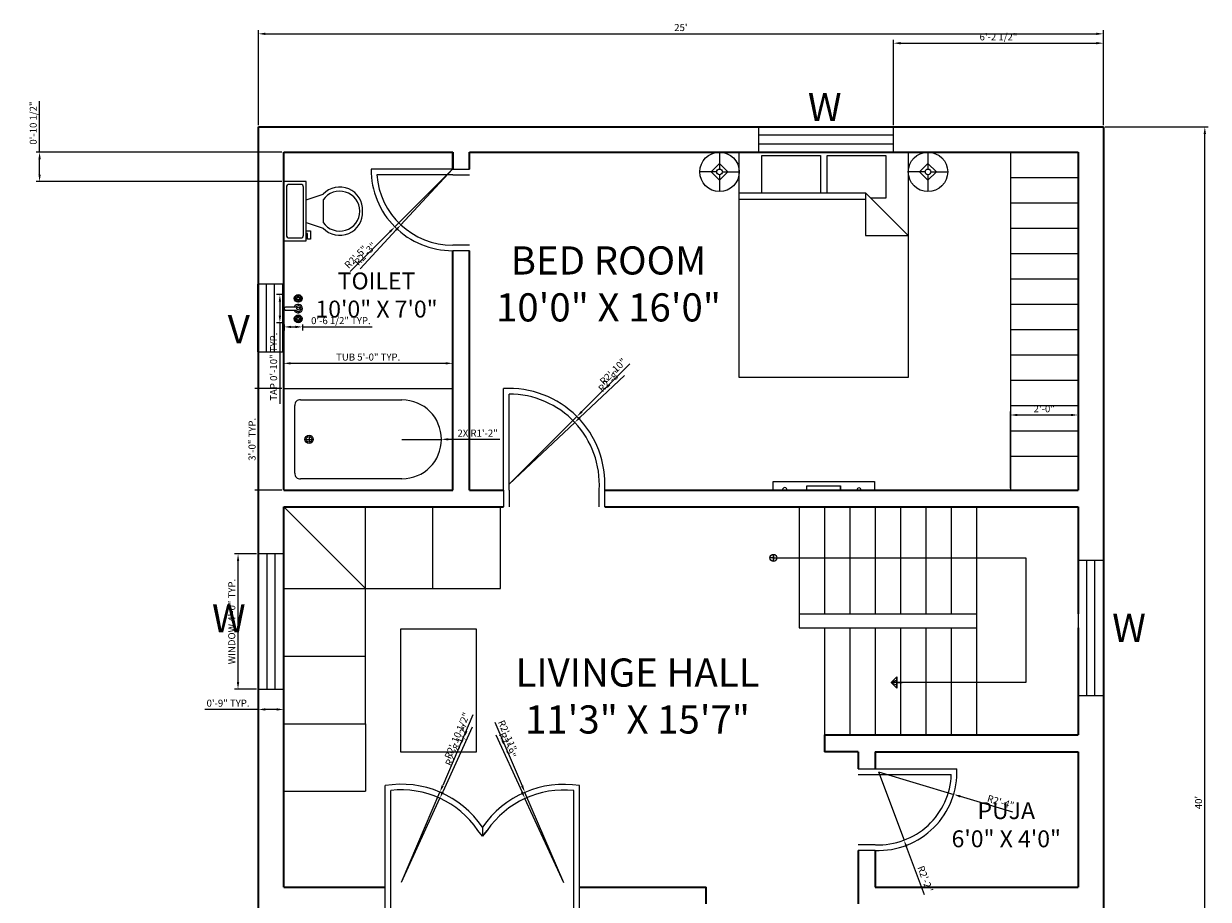
# Model space of a CAD drawing. Units: inches. Extents: x 2318 to 3542, y 1525 to 2117.
# Tile 2 of 6: x 2318 to 2739, y 1758 to 2069. Entities that reach past the tile are written whole.
import ezdxf

# ---------------------------------------------------------------- set-up
doc = ezdxf.new("R2010")
doc.units = ezdxf.units.IN
for name, color, linetype, lineweight in [('A-ANNO-DIMS', 2, 'Continuous', 18), ('A-ANNO-SYMB', 2, 'Continuous', 13), ('A-ANNO-TEXT', 7, 'Continuous', 18), ('A-AREA-IDEN', 7, 'Continuous', 25), ('A-DOOR', 4, 'Continuous', 18), ('A-EQPM', 9, 'Continuous', 18), ('A-FLOR-CASE', 8, 'Continuous', 18), ('A-FLOR-FIXT', 9, 'Continuous', 18), ('A-FLOR-STRS', 3, 'Continuous', 18), ('A-FURN', 8, 'Continuous', 18), ('A-GLAZ', 4, 'Continuous', 18), ('A-WALL', 7, 'Continuous', 35)]:
    doc.layers.add(name, color=color, linetype=linetype, lineweight=lineweight)
doc.styles.add('Annotative', font='arial.ttf')
doc.styles.get("Standard").update_dxf_attribs({"font": 'arial.ttf'})
doc.dimstyles.new('ISO-25', dxfattribs={"dimtxt": 2.5, "dimasz": 2.5, "dimexe": 1.25, "dimexo": 0.625, "dimtad": 1, "dimdec": 0, "dimlunit": 3, "dimtxsty": 'Standard', "dimcen": 2.5, "dimadec": 0, "dimazin": 0, "dimtfac": 1, "dimtdec": 0, "dimtmove": 0, "dimatfit": 3, "dimfxl": 1, "dimarcsym": 0})

# ---------------------------------------------------------------- blocks, each defined once
blk = doc.blocks.new('Bed - Queen')
for p, q in [((0, -80.00003), (0, 0)), ((0, 0), (59.99999, 0)), ((59.99999, 0), (59.99999, -80.00003)), ((7.99999, -1.2), (28.79998, -1.2)), ((7.99999, -14.4), (7.99999, -1.2)), ((28.79998, -1.2), (28.79998, -14.4)), ((31.19999, -1.2), (51.99999, -1.2)), ((31.19999, -14.4), (31.19999, -1.2)), ((51.99999, -1.2), (51.99999, -16.4)), ((0, -14.4), (44.8, -14.4)), ((44.8, -16.8), (0, -16.8)), ((59.99999, -29.6), (44.8, -14.4)), ((44.8, -14.4), (44.8, -29.6)), ((51.99999, -16.4), (46.79936, -16.4)), ((44.8, -29.6), (59.99999, -29.6)), ((59.99999, -80.00003), (0, -80.00003))]:
    blk.add_line(p, q)
blk = doc.blocks.new('Lamp - Table')
for p, q in [((0, 7), (0, 1)), ((-1, 0), (-7, 0)), ((0, 3), (-3, 0)), ((-3, 0), (0, -3)), ((3, 0), (0, 3)), ((0, -3), (3, 0)), ((1, 0), (7, 0)), ((0, -1), (0, -7))]:
    blk.add_line(p, q)
for radius in [7, 1]:
    blk.add_circle((0, 0), radius)
blk = doc.blocks.new('Bath Tub - 26 x 60 in.')
for p, q in [((8, -18), (10, -18)), ((9, -17), (9, -19))]:
    blk.add_line(p, q)
blk.add_lwpolyline([(0, -36), (0, 0), (60, 0), (60, -36)], close=True)
for points in [[(6, -4), (42, -4)], [(4, -30), (4, -6)], [(42, -32), (6, -32)]]:
    blk.add_lwpolyline(points)
for radius in [1.5, 1]:
    blk.add_circle((9, -18), radius)
for centre, radius, start, end in [((5.75, -5.75), 1.77, 81.8699, 188.1301), ((42, -18), 14, 270, 90), ((5.75, -30.25), 1.77, 171.8699, 278.1301)]:
    blk.add_arc(centre, radius, start, end)
blk = doc.blocks.new('Faucet - Bathroom top')
for p, q in [((-4.107, 0.125), (-4.375, 0.125)), ((-3.75, 0.4788), (-3.75, 0.75)), ((-3.5, 0.482), (-3.5, 0.75)), ((-3.1461, 0.125), (-2.875, 0.125)), ((3.143, 0.125), (2.875, 0.125)), ((3.5, 0.4788), (3.5, 0.75)), ((3.75, 0.482), (3.75, 0.75)), ((4.1039, 0.125), (4.375, 0.125)), ((-4.1039, -0.125), (-4.375, -0.125)), ((-3.75, -0.4821), (-3.75, -0.75)), ((-3.5, -0.4789), (-3.5, -0.75)), ((-3.143, -0.125), (-2.875, -0.125)), ((-0.5, -0.8639), (-0.5, -4.5)), ((0.5, -4.5), (0.5, -0.8631)), ((3.1461, -0.125), (2.875, -0.125)), ((3.5, -0.4821), (3.5, -0.75)), ((3.75, -0.4789), (3.75, -0.75)), ((4.107, -0.125), (4.375, -0.125))]:
    blk.add_line(p, q)
for centre, radius in [((-3.625, 0), 1.375), ((-4.625, 0), 0.2795), ((-3.625, 0), 0.5), ((-3.625, 1), 0.2795), ((-2.625, 0), 0.2795), ((0, 0), 0.5), ((3.625, 0), 1.375), ((2.625, 0), 0.2795), ((3.625, 0), 0.5), ((3.625, 1), 0.2795), ((4.625, 0), 0.2795), ((-3.625, -1), 0.2795), ((3.625, -1), 0.2795)]:
    blk.add_circle(centre, radius)
for centre, radius, start, end in [((-3.625, 0), 1, 105.2407, 164.2093), ((-3.625, 0), 1, 16.44125, 74.07887), ((0, 0), 1.5, 289.6514, 250.3603), ((0, 0), 1, 300.3431, 239.7554), ((3.625, 0), 1, 106.12, 164.0884), ((3.625, 0), 1, 16.23422, 73.90469), ((-3.625, 0), 1, 196.2342, 253.9047), ((-3.625, 0), 1, 286.12, 344.0884), ((3.625, 0), 1, 196.4413, 254.0789), ((3.625, 0), 1, 285.2407, 344.2093), ((0, -4.5), 0.5, 180, 0)]:
    blk.add_arc(centre, radius, start, end)
blk = doc.blocks.new('*U14')
for p, q in [((241.3, -152.4), (241.3, -50.8)), ((-203.2, -215.9), (-203.2, -203.2)), ((-177.8, -203.2), (-177.8, -241.3)), ((-101.6, -203.2), (-152.4, -355.6)), ((101.6, -203.2), (152.4, -355.6)), ((-254, -215.9), (-203.2, -215.9)), ((-254, -241.3), (-254, -215.9)), ((-177.8, -241.3), (-254, -241.3)), ((101.6, -355.6), (-101.6, -355.6))]:
    blk.add_line(p, q)
blk.add_lwpolyline([(266.7, -203.2), (266.7, 0), (-266.7, 0), (-266.7, -203.2)], close=True)
for points in [[(-241.3, -50.8), (-241.3, -152.4)], [(215.9, -25.4), (-215.9, -25.4)], [(-215.9, -177.8), (215.9, -177.8)]]:
    blk.add_lwpolyline(points)
for centre, radius, start, end in [((-219.075, -47.625), 22.45064, 81.8699, 188.1301), ((219.075, -47.625), 22.45064, 351.8699, 98.1301), ((-219.075, -155.575), 22.45064, 171.869898, 278.1301), ((219.075, -155.575), 22.45064, 261.8699, 8.1301), ((-12.12088, -505.93752), 205.61935, 133.01722, 273.38), ((0.94996, -504.77674), 181.02486, 124.50543, 269.7), ((-0.94742, -504.77674), 181.02486, 270.3, 55.4946), ((12.12342, -505.93752), 205.61935, 266.62, 46.9828)]:
    blk.add_arc(centre, radius, start, end)
blk = doc.blocks.new('*D15')
at = {"layer": 'A-ANNO-DIMS', "color": 0, "lineweight": -2, "transparency": 16777216}
for p, q in [((2401.66, 2033.24), (2401.66, 2066.9)), ((2404.16, 2065.65), (2699.16, 2065.65)), ((2701.66, 2033.24), (2701.66, 2066.9))]:
    blk.add_line(p, q, dxfattribs=at)
at = {"layer": 'A-ANNO-DIMS', "color": 0, "transparency": 16777216}
for points in [[(2404.16, 2066.06), (2404.16, 2065.23), (2401.66, 2065.65)], [(2699.16, 2066.06), (2699.16, 2065.23), (2701.66, 2065.65)]]:
    blk.add_solid(points, dxfattribs=at)
at = {"layer": 'Defpoints', "color": 0, "transparency": 16777216}
for p in [(2701.66, 2065.65), (2401.66, 2032.62), (2701.66, 2032.62)]:
    blk.add_point(p, dxfattribs=at)
at = {"layer": 'A-ANNO-DIMS', "color": 0, "transparency": 16777216, "insert": (2551.66, 2067.55), "char_height": 2.5, "attachment_point": 5}
blk.add_mtext("25'", dxfattribs=at)
blk = doc.blocks.new('*D16')
at = {"layer": 'A-ANNO-DIMS', "color": 0, "lineweight": -2, "transparency": 16777216}
for p, q in [((2702.28, 2032.62), (2738.91, 2032.62)), ((2737.66, 1555.12), (2737.66, 2030.12)), ((2702.28, 1552.62), (2738.91, 1552.62))]:
    blk.add_line(p, q, dxfattribs=at)
at = {"layer": 'A-ANNO-DIMS', "color": 0, "transparency": 16777216}
for points in [[(2737.24, 2030.12), (2738.07, 2030.12), (2737.66, 2032.62)], [(2737.24, 1555.12), (2738.07, 1555.12), (2737.66, 1552.62)]]:
    blk.add_solid(points, dxfattribs=at)
at = {"layer": 'Defpoints', "color": 0, "transparency": 16777216}
for p in [(2701.66, 2032.62), (2737.66, 2032.62), (2701.66, 1552.62)]:
    blk.add_point(p, dxfattribs=at)
at = {"layer": 'A-ANNO-DIMS', "color": 0, "transparency": 16777216, "insert": (2735.76, 1792.62), "char_height": 2.5, "attachment_point": 5, "rotation": 90}
blk.add_mtext("40'", dxfattribs=at)
blk = doc.blocks.new('WIN-48x9')
for p, q in [((48, 9), (0, 9)), ((0, 9), (0, 0)), ((48, 0), (48, 9)), ((48, 6), (0, 6)), ((0, 3), (48, 3)), ((0, 0), (48, 0))]:
    blk.add_line(p, q)
blk = doc.blocks.new('VENT-24x9')
for p, q in [((0, 24), (0, 0)), ((9, 24), (0, 24)), ((3, 24), (3, 0)), ((6, 0), (6, 24)), ((9, 0), (9, 24)), ((0, 0), (9, 0))]:
    blk.add_line(p, q)
blk = doc.blocks.new('TV-36-WALL')
for p, q in [((0, 0), (0, 3)), ((0, 3), (36, 3)), ((0, 0), (0, 0)), ((0, 0), (24, 0)), ((0, 0), (12, 0)), ((12, 0), (12, 1.44)), ((12, 1.44), (23.97, 1.44)), ((23.97, 1.44), (24, 0)), ((24, 0), (23.97, 1.44)), ((36, 0), (24, 0)), ((36, 3), (36, 0))]:
    blk.add_line(p, q)
for centre, radius in [((4.16, 0), 0.848), ((30.54, 0), 0.733)]:
    blk.add_arc(centre, radius, 360, 180)
blk = doc.blocks.new('*D28')
at = {"layer": 'A-ANNO-DIMS', "color": 0, "lineweight": -2, "transparency": 16777216}
for p, q in [((2401.03, 1880.9), (2393.21, 1880.9)), ((2394.46, 1835.4), (2394.46, 1878.4)), ((2401.03, 1832.9), (2393.21, 1832.9))]:
    blk.add_line(p, q, dxfattribs=at)
at = {"layer": 'A-ANNO-DIMS', "color": 0, "transparency": 16777216}
for points in [[(2394.04, 1878.4), (2394.87, 1878.4), (2394.46, 1880.9)], [(2394.04, 1835.4), (2394.87, 1835.4), (2394.46, 1832.9)]]:
    blk.add_solid(points, dxfattribs=at)
at = {"layer": 'Defpoints', "color": 0, "transparency": 16777216}
for p in [(2394.46, 1880.9), (2401.66, 1880.9), (2401.66, 1832.9)]:
    blk.add_point(p, dxfattribs=at)
at = {"layer": 'A-ANNO-DIMS', "color": 0, "transparency": 16777216, "insert": (2392.54, 1856.9), "char_height": 2.5, "attachment_point": 5, "rotation": 90}
blk.add_mtext('WINDOW 4\'-0" TYP.', dxfattribs=at)
blk = doc.blocks.new('*D29')
at = {"layer": 'A-ANNO-DIMS', "color": 0, "lineweight": -2, "transparency": 16777216}
for p, q in [((2401.66, 1832.27), (2401.66, 1824.45)), ((2410.66, 1832.27), (2410.66, 1824.45)), ((2401.66, 1825.7), (2382.67, 1825.7)), ((2408.16, 1825.7), (2404.16, 1825.7))]:
    blk.add_line(p, q, dxfattribs=at)
at = {"layer": 'A-ANNO-DIMS', "color": 0, "transparency": 16777216}
for points in [[(2404.16, 1826.11), (2404.16, 1825.28), (2401.66, 1825.7)], [(2408.16, 1826.11), (2408.16, 1825.28), (2410.66, 1825.7)]]:
    blk.add_solid(points, dxfattribs=at)
at = {"layer": 'Defpoints', "color": 0, "transparency": 16777216}
for p in [(2401.66, 1832.9), (2410.66, 1832.9), (2401.66, 1825.7)]:
    blk.add_point(p, dxfattribs=at)
at = {"layer": 'A-ANNO-DIMS', "color": 0, "transparency": 16777216, "insert": (2390.91, 1827.6), "char_height": 2.5, "attachment_point": 5}
blk.add_mtext('0\'-9" TYP.', dxfattribs=at)
blk = doc.blocks.new('*D32')
at = {"layer": 'A-ANNO-DIMS', "color": 0, "lineweight": -2, "transparency": 16777216}
for p, q in [((2410.19, 1973.05), (2408.06, 1973.05)), ((2409.31, 1970.55), (2409.31, 1965.55)), ((2410.19, 1963.05), (2408.06, 1963.05)), ((2409.31, 1963.05), (2409.31, 1934.29))]:
    blk.add_line(p, q, dxfattribs=at)
at = {"layer": 'A-ANNO-DIMS', "color": 0, "transparency": 16777216}
for points in [[(2408.9, 1970.55), (2409.73, 1970.55), (2409.31, 1973.05)], [(2408.9, 1965.55), (2409.73, 1965.55), (2409.31, 1963.05)]]:
    blk.add_solid(points, dxfattribs=at)
at = {"layer": 'Defpoints', "color": 0, "transparency": 16777216}
for p in [(2410.81, 1973.05), (2409.31, 1963.05), (2410.81, 1963.05)]:
    blk.add_point(p, dxfattribs=at)
at = {"layer": 'A-ANNO-DIMS', "color": 0, "transparency": 16777216, "insert": (2407.41, 1947.42), "char_height": 2.5, "attachment_point": 5, "rotation": 90}
blk.add_mtext('TAP 0\'-10" TYP.', dxfattribs=at)
blk = doc.blocks.new('*D33')
at = {"layer": 'A-ANNO-DIMS', "color": 0, "lineweight": -2, "transparency": 16777216}
for p, q in [((2410.81, 1962.43), (2410.81, 1960.3)), ((2413.31, 1961.55), (2414.81, 1961.55)), ((2417.31, 1962.43), (2417.31, 1960.3)), ((2417.31, 1961.55), (2442.13, 1961.55))]:
    blk.add_line(p, q, dxfattribs=at)
at = {"layer": 'A-ANNO-DIMS', "color": 0, "transparency": 16777216}
for points in [[(2413.31, 1961.97), (2413.31, 1961.13), (2410.81, 1961.55)], [(2414.81, 1961.97), (2414.81, 1961.13), (2417.31, 1961.55)]]:
    blk.add_solid(points, dxfattribs=at)
at = {"layer": 'Defpoints', "color": 0, "transparency": 16777216}
for p in [(2410.81, 1963.05), (2417.31, 1963.05), (2417.31, 1961.55)]:
    blk.add_point(p, dxfattribs=at)
at = {"layer": 'A-ANNO-DIMS', "color": 0, "transparency": 16777216, "insert": (2430.97, 1963.47), "char_height": 2.5, "attachment_point": 5}
blk.add_mtext('0\'-6 1/2" TYP.', dxfattribs=at)
blk = doc.blocks.new('*D42')
at = {"layer": 'A-ANNO-DIMS', "color": 0, "lineweight": -2, "transparency": 16777216}
for p, q in [((2410.66, 1940.24), (2410.66, 1949.87)), ((2413.16, 1948.62), (2468.16, 1948.62)), ((2470.66, 1940.24), (2470.66, 1949.87))]:
    blk.add_line(p, q, dxfattribs=at)
at = {"layer": 'A-ANNO-DIMS', "color": 0, "transparency": 16777216}
for points in [[(2413.16, 1949.04), (2413.16, 1948.2), (2410.66, 1948.62)], [(2468.16, 1949.04), (2468.16, 1948.2), (2470.66, 1948.62)]]:
    blk.add_solid(points, dxfattribs=at)
at = {"layer": 'Defpoints', "color": 0, "transparency": 16777216}
for p in [(2470.66, 1948.62), (2410.66, 1939.62), (2470.66, 1939.62)]:
    blk.add_point(p, dxfattribs=at)
at = {"layer": 'A-ANNO-DIMS', "color": 0, "transparency": 16777216, "insert": (2440.66, 1950.52), "char_height": 2.5, "attachment_point": 5}
blk.add_mtext('TUB 5\'-0" TYP.', dxfattribs=at)
blk = doc.blocks.new('*D43')
at = {"layer": 'A-ANNO-DIMS', "color": 0, "lineweight": -2, "transparency": 16777216}
for p, q in [((2410.03, 1939.62), (2400.41, 1939.62)), ((2401.66, 1906.12), (2401.66, 1937.12)), ((2410.03, 1903.62), (2400.41, 1903.62))]:
    blk.add_line(p, q, dxfattribs=at)
at = {"layer": 'A-ANNO-DIMS', "color": 0, "transparency": 16777216}
for points in [[(2401.24, 1937.12), (2402.07, 1937.12), (2401.66, 1939.62)], [(2401.24, 1906.12), (2402.07, 1906.12), (2401.66, 1903.62)]]:
    blk.add_solid(points, dxfattribs=at)
at = {"layer": 'Defpoints', "color": 0, "transparency": 16777216}
for p in [(2401.66, 1939.62), (2410.66, 1939.62), (2410.66, 1903.62)]:
    blk.add_point(p, dxfattribs=at)
at = {"layer": 'A-ANNO-DIMS', "color": 0, "transparency": 16777216, "insert": (2399.75, 1921.62), "char_height": 2.5, "attachment_point": 5, "rotation": 90}
blk.add_mtext('3\'-0" TYP.', dxfattribs=at)
blk = doc.blocks.new('*D67')
at = {"layer": 'A-ANNO-DIMS', "color": 0, "lineweight": -2, "transparency": 16777216}
for p, q in [((2668.66, 1904.24), (2668.66, 1931.52)), ((2692.66, 1904.24), (2692.66, 1931.52)), ((2671.16, 1930.27), (2690.16, 1930.27))]:
    blk.add_line(p, q, dxfattribs=at)
at = {"layer": 'A-ANNO-DIMS', "color": 0, "transparency": 16777216}
for points in [[(2671.16, 1930.69), (2671.16, 1929.85), (2668.66, 1930.27)], [(2690.16, 1930.69), (2690.16, 1929.85), (2692.66, 1930.27)]]:
    blk.add_solid(points, dxfattribs=at)
at = {"layer": 'Defpoints', "color": 0, "transparency": 16777216}
for p in [(2692.66, 1930.27), (2668.66, 1903.62), (2692.66, 1903.62)]:
    blk.add_point(p, dxfattribs=at)
at = {"layer": 'A-ANNO-DIMS', "color": 0, "transparency": 16777216, "insert": (2680.66, 1932.17), "char_height": 2.5, "attachment_point": 5}
blk.add_mtext('2\'-0"', dxfattribs=at)
blk = doc.blocks.new('*D71')
at = {"layer": 'A-ANNO-DIMS', "color": 0, "lineweight": -2, "transparency": 16777216}
for p, q in [((2627.17, 2033.24), (2627.17, 2063.57)), ((2629.67, 2062.32), (2699.16, 2062.32)), ((2701.66, 2033.24), (2701.66, 2063.57))]:
    blk.add_line(p, q, dxfattribs=at)
at = {"layer": 'A-ANNO-DIMS', "color": 0, "transparency": 16777216}
for points in [[(2629.67, 2062.74), (2629.67, 2061.91), (2627.17, 2062.32)], [(2699.16, 2062.74), (2699.16, 2061.91), (2701.66, 2062.32)]]:
    blk.add_solid(points, dxfattribs=at)
at = {"layer": 'Defpoints', "color": 0, "transparency": 16777216}
for p in [(2701.66, 2062.32), (2627.17, 2032.62), (2701.66, 2032.62)]:
    blk.add_point(p, dxfattribs=at)
at = {"layer": 'A-ANNO-DIMS', "color": 0, "transparency": 16777216, "insert": (2664.41, 2064.24), "char_height": 2.5, "attachment_point": 5}
blk.add_mtext('6\'-2 1/2"', dxfattribs=at)
blk = doc.blocks.new('*D74')
at = {"layer": 'A-ANNO-DIMS', "color": 0, "lineweight": -2, "transparency": 16777216}
for p, q in [((2324.01, 2023.62), (2324.01, 2041.78)), ((2410.03, 2023.62), (2322.76, 2023.62)), ((2324.01, 2015.67), (2324.01, 2021.12)), ((2410.03, 2013.17), (2322.76, 2013.17))]:
    blk.add_line(p, q, dxfattribs=at)
at = {"layer": 'A-ANNO-DIMS', "color": 0, "transparency": 16777216}
for points in [[(2323.59, 2021.12), (2324.42, 2021.12), (2324.01, 2023.62)], [(2323.59, 2015.67), (2324.42, 2015.67), (2324.01, 2013.17)]]:
    blk.add_solid(points, dxfattribs=at)
at = {"layer": 'Defpoints', "color": 0, "transparency": 16777216}
for p in [(2324.01, 2023.62), (2410.66, 2023.62), (2410.66, 2013.17)]:
    blk.add_point(p, dxfattribs=at)
at = {"layer": 'A-ANNO-DIMS', "color": 0, "transparency": 16777216, "insert": (2322.09, 2033.95), "char_height": 2.5, "attachment_point": 5, "rotation": 90}
blk.add_mtext('0\'-10 1/2"', dxfattribs=at)
blk = doc.blocks.new('*D76')
at = {"layer": 'A-ANNO-DIMS', "color": 0, "lineweight": -2, "transparency": 16777216}
for p, q in [((2533.51, 1948.47), (2516.53, 1931.49)), ((2490.71, 1905.68), (2514.76, 1929.72))]:
    blk.add_line(p, q, dxfattribs=at)
at = {"layer": 'A-ANNO-DIMS', "color": 0, "transparency": 16777216}
blk.add_solid([(2516.23, 1931.78), (2516.82, 1931.19), (2514.76, 1929.72)], dxfattribs=at)
at = {"layer": 'Defpoints', "color": 0, "transparency": 16777216}
for p in [(2514.76, 1929.72), (2490.71, 1905.68)]:
    blk.add_point(p, dxfattribs=at)
at = {"layer": 'A-ANNO-DIMS', "color": 0, "transparency": 16777216, "insert": (2527.84, 1945.49), "char_height": 2.5, "attachment_point": 5, "rotation": 44.9996}
blk.add_mtext('R2\'-10"', dxfattribs=at)
blk = doc.blocks.new('*D77')
at = {"layer": 'A-ANNO-DIMS', "color": 0, "lineweight": -2, "transparency": 16777216}
for p, q in [((2470.58, 2017.54), (2450.13, 1997.09)), ((2434.22, 1981.18), (2448.36, 1995.32))]:
    blk.add_line(p, q, dxfattribs=at)
at = {"layer": 'A-ANNO-DIMS', "color": 0, "transparency": 16777216}
blk.add_solid([(2448.06, 1995.62), (2448.65, 1995.03), (2450.13, 1997.09)], dxfattribs=at)
at = {"layer": 'Defpoints', "color": 0, "transparency": 16777216}
for p in [(2470.58, 2017.54), (2450.13, 1997.09)]:
    blk.add_point(p, dxfattribs=at)
at = {"layer": 'A-ANNO-DIMS', "color": 0, "transparency": 16777216, "insert": (2436.51, 1986.16), "char_height": 2.5, "attachment_point": 5, "rotation": 45.0005}
blk.add_mtext('R2\'-5"', dxfattribs=at)
blk = doc.blocks.new('*D78')
at = {"layer": 'A-ANNO-DIMS', "color": 0, "lineweight": -2, "transparency": 16777216}
for p, q in [((2621.77, 1803.51), (2648.51, 1795.51)), ((2669.48, 1789.24), (2650.9, 1794.8))]:
    blk.add_line(p, q, dxfattribs=at)
at = {"layer": 'A-ANNO-DIMS', "color": 0, "transparency": 16777216}
blk.add_solid([(2651.02, 1795.2), (2650.79, 1794.4), (2648.51, 1795.51)], dxfattribs=at)
at = {"layer": 'Defpoints', "color": 0, "transparency": 16777216}
for p in [(2621.77, 1803.51), (2648.51, 1795.51)]:
    blk.add_point(p, dxfattribs=at)
at = {"layer": 'A-ANNO-DIMS', "color": 0, "transparency": 16777216, "insert": (2665.09, 1792.52), "char_height": 2.5, "attachment_point": 5, "rotation": 343.3554}
blk.add_mtext('R2\'-4"', dxfattribs=at)
blk = doc.blocks.new('*D79')
at = {"layer": 'A-ANNO-DIMS', "color": 0, "lineweight": -2, "transparency": 16777216}
for p, q in [((2477.84, 1823.8), (2467.1, 1798.63)), ((2452.49, 1764.38), (2466.12, 1796.33))]:
    blk.add_line(p, q, dxfattribs=at)
at = {"layer": 'A-ANNO-DIMS', "color": 0, "transparency": 16777216}
blk.add_solid([(2466.72, 1798.79), (2467.48, 1798.46), (2466.12, 1796.33)], dxfattribs=at)
at = {"layer": 'Defpoints', "color": 0, "transparency": 16777216}
for p in [(2466.12, 1796.33), (2452.49, 1764.38)]:
    blk.add_point(p, dxfattribs=at)
at = {"layer": 'A-ANNO-DIMS', "color": 0, "transparency": 16777216, "insert": (2472.53, 1816.25), "char_height": 2.5, "attachment_point": 5, "rotation": 66.8971}
blk.add_mtext('R2\'-10 1/2"', dxfattribs=at)
blk = doc.blocks.new('*D80')
at = {"layer": 'A-ANNO-DIMS', "color": 0, "lineweight": -2, "transparency": 16777216}
for p, q in [((2485.64, 1821.13), (2495.32, 1798.54)), ((2510.07, 1764.13), (2496.3, 1796.24))]:
    blk.add_line(p, q, dxfattribs=at)
at = {"layer": 'A-ANNO-DIMS', "color": 0, "transparency": 16777216}
blk.add_solid([(2495.7, 1798.7), (2494.94, 1798.38), (2496.3, 1796.24)], dxfattribs=at)
at = {"layer": 'Defpoints', "color": 0, "transparency": 16777216}
for p in [(2496.3, 1796.24), (2510.07, 1764.13)]:
    blk.add_point(p, dxfattribs=at)
at = {"layer": 'A-ANNO-DIMS', "color": 0, "transparency": 16777216, "insert": (2489.77, 1816.25), "char_height": 2.5, "attachment_point": 5, "rotation": 293.2052}
blk.add_mtext('R2\'-11"', dxfattribs=at)
blk = doc.blocks.new('*D96')
at = {"layer": 'A-ANNO-DIMS', "color": 0, "lineweight": -2, "transparency": 16777216}
for p, q in [((2485.92, 1816.69), (2495.28, 1796.33)), ((2510.07, 1764.13), (2496.32, 1794.06))]:
    blk.add_line(p, q, dxfattribs=at)
at = {"layer": 'A-ANNO-DIMS', "color": 0, "transparency": 16777216}
blk.add_solid([(2495.65, 1796.51), (2494.9, 1796.16), (2496.32, 1794.06)], dxfattribs=at)
at = {"layer": 'Defpoints', "color": 0, "transparency": 16777216}
for p in [(2496.32, 1794.06), (2510.07, 1764.13)]:
    blk.add_point(p, dxfattribs=at)
at = {"layer": 'A-ANNO-DIMS', "color": 0, "transparency": 16777216, "insert": (2489.8, 1812.81), "char_height": 2.5, "attachment_point": 5, "rotation": 294.6786}
blk.add_mtext('R2\'-9"', dxfattribs=at)
blk = doc.blocks.new('*D97')
at = {"layer": 'A-ANNO-DIMS', "color": 0, "lineweight": -2, "transparency": 16777216}
for p, q in [((2477.62, 1819.34), (2467.14, 1796.42)), ((2452.49, 1764.38), (2466.1, 1794.15))]:
    blk.add_line(p, q, dxfattribs=at)
at = {"layer": 'A-ANNO-DIMS', "color": 0, "transparency": 16777216}
blk.add_solid([(2466.76, 1796.59), (2467.52, 1796.25), (2466.1, 1794.15)], dxfattribs=at)
at = {"layer": 'Defpoints', "color": 0, "transparency": 16777216}
for p in [(2466.1, 1794.15), (2452.49, 1764.38)]:
    blk.add_point(p, dxfattribs=at)
at = {"layer": 'A-ANNO-DIMS', "color": 0, "transparency": 16777216, "insert": (2472.53, 1812.81), "char_height": 2.5, "attachment_point": 5, "rotation": 65.4263}
blk.add_mtext('R2\'-8 1/2"', dxfattribs=at)
blk = doc.blocks.new('*D98')
at = {"layer": 'A-ANNO-DIMS', "color": 0, "lineweight": -2, "transparency": 16777216}
for p, q in [((2531.71, 1944.34), (2515.82, 1929.35)), ((2490.71, 1905.68), (2514, 1927.63))]:
    blk.add_line(p, q, dxfattribs=at)
at = {"layer": 'A-ANNO-DIMS', "color": 0, "transparency": 16777216}
blk.add_solid([(2515.53, 1929.65), (2516.1, 1929.04), (2514, 1927.63)], dxfattribs=at)
at = {"layer": 'Defpoints', "color": 0, "transparency": 16777216}
for p in [(2514, 1927.63), (2490.71, 1905.68)]:
    blk.add_point(p, dxfattribs=at)
at = {"layer": 'A-ANNO-DIMS', "color": 0, "transparency": 16777216, "insert": (2526.67, 1942.19), "char_height": 2.5, "attachment_point": 5, "rotation": 43.317}
blk.add_mtext('R2\'-8"', dxfattribs=at)
blk = doc.blocks.new('*D99')
at = {"layer": 'A-ANNO-DIMS', "color": 0, "lineweight": -2, "transparency": 16777216}
for p, q in [((2452.66, 1921.62), (2466.66, 1921.62)), ((2487.36, 1921.62), (2469.16, 1921.62))]:
    blk.add_line(p, q, dxfattribs=at)
at = {"layer": 'A-ANNO-DIMS', "color": 0, "transparency": 16777216}
blk.add_solid([(2469.16, 1922.04), (2469.16, 1921.2), (2466.66, 1921.62)], dxfattribs=at)
at = {"layer": 'Defpoints', "color": 0, "transparency": 16777216}
for p in [(2452.66, 1921.62), (2466.66, 1921.62)]:
    blk.add_point(p, dxfattribs=at)
at = {"layer": 'A-ANNO-DIMS', "color": 0, "transparency": 16777216, "insert": (2479.51, 1923.5), "char_height": 2.5, "attachment_point": 5, "rotation": 0.0007}
blk.add_mtext('2X R1\'-2"', dxfattribs=at)
blk = doc.blocks.new('*D106')
at = {"layer": 'A-ANNO-DIMS', "color": 0, "lineweight": -2, "transparency": 16777216}
for p, q in [((2470.58, 2017.54), (2452.26, 1997.81)), ((2437.77, 1982.2), (2450.56, 1995.98))]:
    blk.add_line(p, q, dxfattribs=at)
at = {"layer": 'A-ANNO-DIMS', "color": 0, "transparency": 16777216}
blk.add_solid([(2450.25, 1996.26), (2450.86, 1995.7), (2452.26, 1997.81)], dxfattribs=at)
at = {"layer": 'Defpoints', "color": 0, "transparency": 16777216}
for p in [(2470.58, 2017.54), (2452.26, 1997.81)]:
    blk.add_point(p, dxfattribs=at)
at = {"layer": 'A-ANNO-DIMS', "color": 0, "transparency": 16777216, "insert": (2439.88, 1987.27), "char_height": 2.5, "attachment_point": 5, "rotation": 47.1246}
blk.add_mtext('R2\'-3"', dxfattribs=at)
blk = doc.blocks.new('*D107')
at = {"layer": 'A-ANNO-DIMS', "color": 0, "lineweight": -2, "transparency": 16777216}
for p, q in [((2621.77, 1803.51), (2630.88, 1779.25)), ((2638.16, 1759.88), (2631.76, 1776.91))]:
    blk.add_line(p, q, dxfattribs=at)
at = {"layer": 'A-ANNO-DIMS', "color": 0, "transparency": 16777216}
blk.add_solid([(2632.15, 1777.06), (2631.37, 1776.76), (2630.88, 1779.25)], dxfattribs=at)
at = {"layer": 'Defpoints', "color": 0, "transparency": 16777216}
for p in [(2621.77, 1803.51), (2630.88, 1779.25)]:
    blk.add_point(p, dxfattribs=at)
at = {"layer": 'A-ANNO-DIMS', "color": 0, "transparency": 16777216, "insert": (2638.11, 1765.36), "char_height": 2.5, "attachment_point": 5, "rotation": 290.5896}
blk.add_mtext('R2\'-2"', dxfattribs=at)

msp = doc.modelspace()

# ---------------------------------------------------------------- linework, layer by layer
at = {"layer": 'A-ANNO-SYMB'}
for p, q in [((2584.5, 1879.53), (2584.5, 1880.77)), ((2584.5, 1880.77), (2584.5, 1879.53)), ((2584.5, 1879.53), (2583.26, 1879.53)), ((2584.5, 1879.53), (2674.13, 1879.53)), ((2584.5, 1879.53), (2584.5, 1878.3)), ((2584.5, 1878.3), (2584.5, 1879.53)), ((2674.13, 1879.53), (2674.13, 1835.26)), ((2626.28, 1835.26), (2628.28, 1837.26)), ((2626.28, 1835.26), (2628.28, 1836.11)), ((2628.28, 1836.11), (2626.28, 1835.26)), ((2628.28, 1835.26), (2626.28, 1835.26)), ((2628.28, 1833.26), (2626.28, 1835.26)), ((2626.28, 1835.26), (2628.28, 1834.26)), ((2628.28, 1835.26), (2628.28, 1837.26)), ((2628.28, 1837.26), (2628.28, 1835.26)), ((2628.28, 1837.26), (2628.28, 1833.26)), ((2629.66, 1835.26), (2628.28, 1835.26)), ((2628.28, 1835.26), (2630.28, 1835.26)), ((2628.28, 1835.26), (2628.28, 1833.26)), ((2628.28, 1833.26), (2628.28, 1835.26)), ((2674.13, 1835.26), (2629.66, 1835.26)), ((2481.24, 1783.87), (2481.24, 1780.63)), ((2481.24, 1780.63), (2479.59, 1782.74)), ((2481.24, 1780.63), (2482.89, 1782.74)), ((2482.89, 1782.74), (2481.24, 1780.63))]:
    msp.add_line(p, q, dxfattribs=at)
msp.add_circle((2584.5, 1879.53), 1.24, dxfattribs=at)
at = {"layer": 'A-DOOR'}
for p, q in [((2470.66, 2017.62), (2441.66, 2017.62)), ((2470.66, 2015.62), (2443.72, 2015.62)), ((2470.66, 2017.62), (2476.66, 2017.62)), ((2470.66, 2015.62), (2476.66, 2015.62)), ((2476.66, 1990.62), (2470.66, 1990.62)), ((2476.66, 1988.62), (2470.66, 1988.62)), ((2488.66, 1903.62), (2488.66, 1939.62)), ((2490.66, 1903.62), (2490.66, 1937.68)), ((2488.66, 1903.62), (2488.66, 1897.62)), ((2490.66, 1903.62), (2490.66, 1897.62)), ((2522.66, 1897.62), (2522.66, 1903.62)), ((2524.66, 1897.62), (2524.66, 1903.62)), ((2614.66, 1804.62), (2620.66, 1804.62)), ((2614.66, 1804.62), (2620.66, 1804.62)), ((2620.66, 1804.62), (2649.66, 1804.62)), ((2614.66, 1802.62), (2620.66, 1802.62)), ((2620.66, 1802.62), (2647.66, 1802.62)), ((2446.66, 1762.62), (2446.66, 1798.62)), ((2448.66, 1762.62), (2448.66, 1796.89)), ((2513.66, 1762.62), (2513.66, 1796.87)), ((2515.66, 1762.62), (2515.66, 1798.62)), ((2620.66, 1777.62), (2614.66, 1777.62)), ((2620.66, 1775.62), (2614.66, 1775.62)), ((2446.66, 1753.62), (2446.66, 1762.62)), ((2448.66, 1753.62), (2448.66, 1762.62)), ((2513.66, 1753.62), (2513.66, 1762.62)), ((2515.66, 1753.62), (2515.66, 1762.62))]:
    msp.add_line(p, q, dxfattribs=at)
for centre, radius, start, end in [((2470.58, 2017.54), 28.92, 179.8408, 270.1592), ((2470.58, 2017.54), 26.92, 184.0892, 270.1592), ((2490.71, 1905.68), 34.01, 356.5317, 93.4683), ((2490.71, 1905.68), 32.01, 356.5317, 90.1024), ((2621.77, 1803.51), 27.91, 267.716, 2.284), ((2621.77, 1803.51), 25.91, 267.716, 358.0366), ((2452.49, 1764.38), 34.74, 34.131, 99.6642), ((2452.49, 1764.38), 32.74, 34.131, 96.7211), ((2510.07, 1764.13), 34.94, 80.7991, 145.6096), ((2510.07, 1764.13), 32.94, 83.7492, 145.6096)]:
    msp.add_arc(centre, radius, start, end, dxfattribs=at)
at = {"layer": 'A-EQPM'}
for p, q in [((2572.39, 1903.62), (2584.39, 1903.62)), ((2632.39, 1903.62), (2620.39, 1903.62))]:
    msp.add_line(p, q, dxfattribs=at)
at = {"layer": 'A-FLOR-CASE'}
for p, q in [((2668.66, 2023.62), (2668.66, 1903.62)), ((2668.66, 2014.62), (2692.66, 2014.62)), ((2668.66, 2005.62), (2692.66, 2005.62)), ((2668.66, 1996.62), (2692.66, 1996.62)), ((2668.66, 1987.62), (2692.66, 1987.62)), ((2668.66, 1978.62), (2692.66, 1978.62)), ((2668.66, 1969.62), (2692.66, 1969.62)), ((2668.66, 1960.62), (2692.66, 1960.62)), ((2668.66, 1951.62), (2692.66, 1951.62)), ((2668.66, 1942.62), (2692.66, 1942.62)), ((2668.66, 1933.62), (2692.66, 1933.62)), ((2668.66, 1924.62), (2692.66, 1924.62)), ((2668.66, 1915.62), (2692.66, 1915.62))]:
    msp.add_line(p, q, dxfattribs=at)
at = {"layer": 'A-FLOR-STRS'}
for p, q in [((2593.66, 1897.62), (2593.66, 1854.62)), ((2602.66, 1897.62), (2602.66, 1859.62)), ((2611.66, 1897.62), (2611.66, 1859.62)), ((2620.66, 1897.62), (2620.66, 1859.62)), ((2629.66, 1897.62), (2629.66, 1859.62)), ((2638.66, 1897.62), (2638.66, 1859.62)), ((2647.66, 1897.62), (2647.66, 1859.62)), ((2656.66, 1897.62), (2656.66, 1859.62)), ((2593.66, 1859.62), (2656.66, 1859.62)), ((2656.66, 1859.62), (2656.66, 1854.62)), ((2593.66, 1854.62), (2656.66, 1854.62)), ((2602.66, 1854.62), (2602.66, 1816.62)), ((2611.66, 1854.62), (2611.66, 1816.62)), ((2620.66, 1854.62), (2620.66, 1816.62)), ((2629.66, 1854.62), (2629.66, 1816.62)), ((2638.66, 1854.62), (2638.66, 1816.62)), ((2647.66, 1854.62), (2647.66, 1816.62)), ((2656.66, 1854.62), (2656.66, 1816.62))]:
    msp.add_line(p, q, dxfattribs=at)
at = {"layer": 'A-FURN'}
for p, q in [((2410.66, 1897.62), (2439.66, 1868.62)), ((2439.66, 1820.62), (2439.66, 1897.62)), ((2463.66, 1868.62), (2463.66, 1897.62)), ((2487.66, 1868.62), (2487.66, 1897.62)), ((2410.66, 1868.62), (2487.66, 1868.62)), ((2410.66, 1844.62), (2439.66, 1844.62)), ((2410.66, 1820.62), (2439.66, 1820.62)), ((2439.66, 1820.62), (2439.66, 1796.62)), ((2410.66, 1796.62), (2439.66, 1796.62))]:
    msp.add_line(p, q, dxfattribs=at)
msp.add_lwpolyline([(2452.3, 1810.49), (2452.3, 1854.27), (2479.03, 1854.27), (2479.03, 1810.49)], close=True, dxfattribs=at)
at = {"layer": 'A-WALL'}
for p, q in [((2401.66, 2032.62), (2701.66, 2032.62)), ((2401.66, 1552.62), (2401.66, 2032.62)), ((2701.66, 2032.62), (2701.66, 1552.62)), ((2410.66, 2023.62), (2470.66, 2023.62)), ((2410.66, 1903.62), (2410.66, 2023.62)), ((2470.66, 2023.62), (2470.66, 2017.62)), ((2470.66, 2017.62), (2470.66, 2023.62)), ((2476.66, 2023.62), (2692.66, 2023.62)), ((2476.66, 2017.62), (2476.66, 2023.62)), ((2692.66, 2023.62), (2692.66, 1903.62)), ((2470.66, 1903.62), (2470.66, 1988.62)), ((2476.66, 1903.62), (2476.66, 1988.62)), ((2410.66, 1903.62), (2470.66, 1903.62)), ((2476.66, 1903.62), (2488.66, 1903.62)), ((2476.66, 1903.62), (2488.66, 1903.62)), ((2476.66, 1903.62), (2488.66, 1903.62)), ((2524.66, 1903.62), (2692.66, 1903.62)), ((2410.66, 1897.62), (2488.66, 1897.62)), ((2410.66, 1762.62), (2410.66, 1897.62)), ((2524.66, 1897.62), (2692.66, 1897.62)), ((2692.66, 1897.62), (2692.66, 1859.62)), ((2692.66, 1854.62), (2692.66, 1816.62)), ((2602.66, 1816.62), (2692.66, 1816.62)), ((2602.66, 1816.62), (2602.66, 1810.62)), ((2614.66, 1810.62), (2602.66, 1810.62)), ((2614.66, 1810.62), (2614.66, 1804.62)), ((2614.66, 1810.62), (2614.66, 1804.62)), ((2620.66, 1810.62), (2620.66, 1804.62)), ((2620.66, 1810.62), (2692.66, 1810.62)), ((2692.66, 1810.62), (2692.66, 1762.62)), ((2614.66, 1775.62), (2614.66, 1762.62)), ((2620.66, 1775.62), (2620.66, 1762.62)), ((2410.66, 1762.62), (2446.66, 1762.62)), ((2515.66, 1762.62), (2560.66, 1762.62)), ((2560.66, 1756.62), (2560.66, 1762.62)), ((2614.66, 1762.62), (2614.66, 1756.62)), ((2620.66, 1762.62), (2692.66, 1762.62))]:
    msp.add_line(p, q, dxfattribs=at)

# ---------------------------------------------------------------- block references
at = {"layer": 'A-EQPM'}
msp.add_blockref('TV-36-WALL', (2584.39, 1903.62), dxfattribs=at)
at = {"layer": 'A-FLOR-FIXT', "xscale": 0.0393700787401575, "yscale": 0.0393700787401575, "zscale": 0.0393700787401575, "rotation": 90}
msp.add_blockref('*U14', (2410.66, 2002.67), dxfattribs=at)
at = {"layer": 'A-FLOR-FIXT', "rotation": 270}
msp.add_blockref('Faucet - Bathroom top', (2415.81, 1968.05), dxfattribs=at)
at = {"layer": 'A-FLOR-FIXT'}
msp.add_blockref('Bath Tub - 26 x 60 in.', (2410.66, 1939.62), dxfattribs=at)
at = {"layer": 'A-FURN'}
for name, p in [('Lamp - Table', (2565.39, 2016.62)), ('Bed - Queen', (2572.39, 2023.62)), ('Lamp - Table', (2639.39, 2016.62))]:
    msp.add_blockref(name, p, dxfattribs=at)
at = {"layer": 'A-GLAZ'}
for name, p in [('WIN-48x9', (2579.17, 2023.62)), ('VENT-24x9', (2401.4, 1952.73))]:
    msp.add_blockref(name, p, dxfattribs=at)
for p, rotation in [((2410.66, 1832.9), 89.99999999999982), ((2701.66, 1830.62), 90.00000000000081)]:
    msp.add_blockref('WIN-48x9', p, dxfattribs=dict(at, rotation=rotation))

# ---------------------------------------------------------------- texts
at = {"layer": 'A-ANNO-TEXT', "char_height": 10, "attachment_point": 1}
for s, insert in [('\\pxt1;W', (2596.74, 2044.65)), ('\\pxt1;V', (2390.8, 1965.74)), ('\\pxt1;W', (2385.2, 1863.04)), ('\\pxt1;W', (2704.77, 1859.68))]:
    msp.add_mtext_dynamic_manual_height_columns(s, width=219.3474, gutter_width=12.5, heights=[0], dxfattribs=dict(at, insert=insert))
at = {"layer": 'A-AREA-IDEN', "char_height": 10, "width": 132.7792, "attachment_point": 1, "style": 'Annotative'}
for s, insert in [('\\pxqc;BED ROOM\\P10\'0" X 16\'0"', (2459.59, 1990.16)), ('\\pxqc;LIVINGE HALL\\P11\'3" X 15\'7"', (2469.88, 1843.79))]:
    msp.add_mtext(s, dxfattribs=dict(at, insert=insert))
at = {"layer": 'A-AREA-IDEN', "char_height": 6, "attachment_point": 1}
for s, insert in [('\\pxqc,t2;TOILET\\P10\'0" X 7\'0"', (2420.2, 1980.89)), ('\\pxqc,t2;PUJA \\P6\'0" X 4\'0"', (2643.76, 1792.74))]:
    msp.add_mtext_dynamic_manual_height_columns(s, width=46.835, gutter_width=12.5, heights=[0], dxfattribs=dict(at, insert=insert))

# ---------------------------------------------------------------- dimensions: what is measured, and where the dimension line sits
at = {"layer": 'A-ANNO-DIMS'}
for base, p1, p2, override, picture, middle in [((2701.66, 2065.65), (2401.66, 2032.62), (2701.66, 2032.62), {"dimclrd": 0, "dimclre": 0, "dimclrt": 0}, '*D15', (2551.66, 2067.55)), ((2701.66, 2062.32), (2627.17, 2032.62), (2701.66, 2032.62), {"dimdec": 1, "dimlfac": 1, "dimrnd": 0, "dimzin": 1, "dimdsep": 46, "dimlunit": 4, "dimfrac": 2}, '*D71', (2664.41, 2064.24)), ((2692.66, 1930.27), (2668.66, 1903.62), (2692.66, 1903.62), {"dimdec": 1, "dimlfac": 1, "dimrnd": 0, "dimzin": 1, "dimdsep": 46, "dimlunit": 4, "dimfrac": 2}, '*D67', (2680.66, 1932.17))]:
    dim = msp.add_linear_dim(base=base, p1=p1, p2=p2, dimstyle='ISO-25', override=override, dxfattribs=at)
    dim.commit()
    dim.dimension.update_dxf_attribs({"geometry": picture, "text_midpoint": middle})
for base, p1, p2, override, picture, middle in [((2324.0065, 2023.6188), (2410.6565, 2013.1739), (2410.6565, 2023.6188), {"dimdec": 1, "dimlfac": 1, "dimrnd": 0, "dimzin": 1, "dimdsep": 46, "dimlunit": 4, "dimfrac": 2}, '*D74', (2322.0889, 2033.9505)), ((2737.66, 2032.62), (2701.66, 1552.62), (2701.66, 2032.62), {"dimclrd": 0, "dimclre": 0, "dimclrt": 0}, '*D16', (2735.76, 1792.62))]:
    dim = msp.add_linear_dim(base=base, p1=p1, p2=p2, angle=90, dimstyle='ISO-25', override=override, dxfattribs=at)
    dim.commit()
    dim.dimension.update_dxf_attribs({"geometry": picture, "text_midpoint": middle})
for center, mpoint, picture, middle in [((2470.58, 2017.54), (2450.13, 1997.09), '*D77', (2437.86, 1984.82)), ((2470.58, 2017.54), (2452.26, 1997.81), '*D106', (2441.27, 1985.97)), ((2490.71, 1905.68), (2514.76, 1929.72), '*D76', (2529.19, 1944.15)), ((2490.71, 1905.68), (2514, 1927.63), '*D98', (2527.97, 1940.81)), ((2452.49, 1764.38), (2466.12, 1796.33), '*D79', (2474.3, 1815.5)), ((2510.07, 1764.13), (2496.3, 1796.24), '*D80', (2488.05, 1815.51)), ((2452.49, 1764.38), (2466.1, 1794.15), '*D97', (2474.27, 1812.01)), ((2510.07, 1764.13), (2496.32, 1794.06), '*D96', (2488.07, 1812.02)), ((2621.77, 1803.51), (2648.51, 1795.51), '*D78', (2664.55, 1790.72)), ((2621.77, 1803.51), (2630.88, 1779.25), '*D107', (2636.35, 1764.7))]:
    dim = msp.add_radius_dim(center=center, mpoint=mpoint, dimstyle='ISO-25', override={"dimdec": 1, "dimlfac": 1, "dimrnd": 0, "dimzin": 1, "dimdsep": 46, "dimlunit": 4, "dimfrac": 2}, dxfattribs=at)
    dim.commit()
    dim.dimension.update_dxf_attribs({"geometry": picture, "text_midpoint": middle, "dimtype": 164})
for base, p1, p2, angle, text, picture, middle in [((2409.31, 1963.05), (2410.81, 1973.05), (2410.81, 1963.05), 270, 'TAP <> TYP.', '*D32', (2407.41, 1947.42)), ((2401.66, 1939.62), (2410.66, 1903.62), (2410.66, 1939.62), 90, '<> TYP.', '*D43', (2399.75, 1921.62)), ((2394.46, 1880.9), (2401.66, 1832.9), (2401.66, 1880.9), 90, 'WINDOW <> TYP.', '*D28', (2392.54, 1856.9)), ((2401.66, 1825.7), (2410.66, 1832.9), (2401.66, 1832.9), 180, '<> TYP.', '*D29', (2390.91, 1827.6))]:
    dim = msp.add_linear_dim(base=base, p1=p1, p2=p2, angle=angle, text=text, dimstyle='ISO-25', override={"dimdec": 1, "dimlfac": 1, "dimrnd": 0, "dimzin": 1, "dimdsep": 46, "dimlunit": 4, "dimfrac": 2}, dxfattribs=at)
    dim.commit()
    dim.dimension.update_dxf_attribs({"geometry": picture, "text_midpoint": middle})
for base, p1, p2, text, picture, middle in [((2417.31, 1961.55), (2410.81, 1963.05), (2417.31, 1963.05), '<> TYP.', '*D33', (2430.97, 1963.47)), ((2470.66, 1948.62), (2410.66, 1939.62), (2470.66, 1939.62), 'TUB <> TYP.', '*D42', (2440.66, 1950.52))]:
    dim = msp.add_linear_dim(base=base, p1=p1, p2=p2, text=text, dimstyle='ISO-25', override={"dimdec": 1, "dimlfac": 1, "dimrnd": 0, "dimzin": 1, "dimdsep": 46, "dimlunit": 4, "dimfrac": 2}, dxfattribs=at)
    dim.commit()
    dim.dimension.update_dxf_attribs({"geometry": picture, "text_midpoint": middle})
dim = msp.add_radius_dim(center=(2452.66, 1921.62), mpoint=(2466.66, 1921.62), text='2X <>', dimstyle='ISO-25', override={"dimdec": 1, "dimlfac": 1, "dimrnd": 0, "dimzin": 1, "dimdsep": 46, "dimlunit": 4, "dimfrac": 2}, dxfattribs=at)
dim.commit()
dim.dimension.update_dxf_attribs({"geometry": '*D99', "text_midpoint": (2479.51, 1923.5)})

doc.saveas('drawing.dxf')
